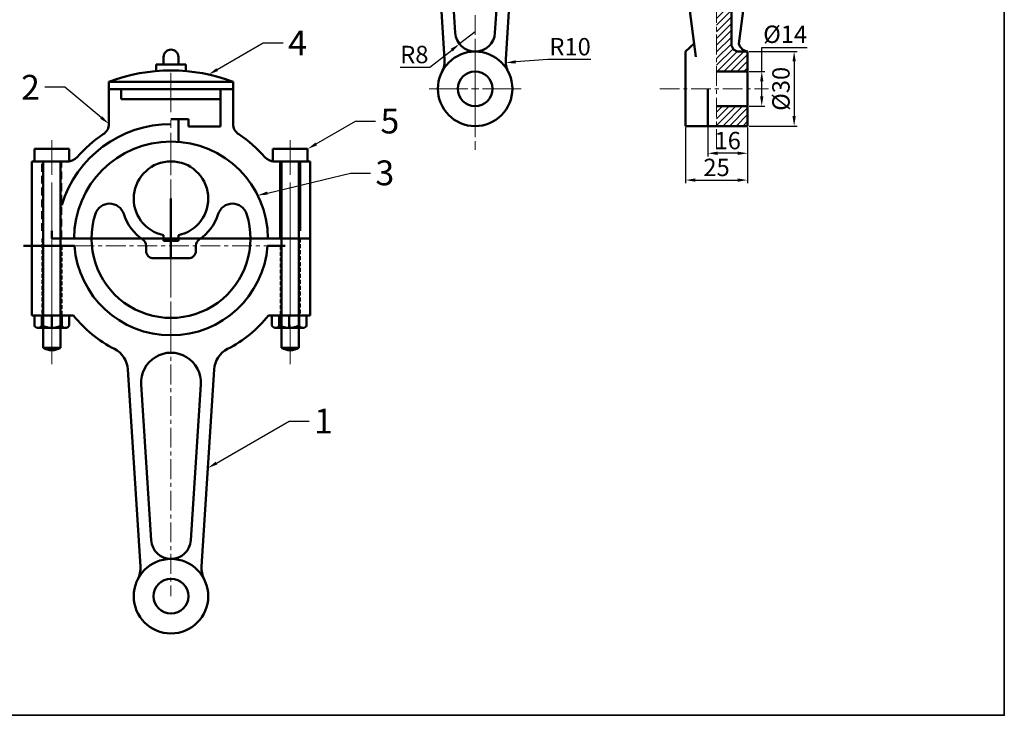
# Model space of a CAD drawing. Units: millimetres. Extents: x 214 to 813, y -258 to 321.
# Tile 2 of 4: x 416 to 813, y -258 to 22. Entities that reach past the tile are written whole.
import ezdxf
from ezdxf import colors
from ezdxf.entities.mleader import LeaderData, LeaderLine
from ezdxf.math import Vec2, Vec3

# ---------------------------------------------------------------- set-up
doc = ezdxf.new("R2010")
doc.units = ezdxf.units.MM
doc.header["$LTSCALE"] = 0.5
doc.linetypes.add('CENTER', pattern=[50.8, 31.75, -6.35, 6.35, -6.35])
doc.linetypes.add('HIDDEN', pattern=[9.525, 6.35, -3.175])
for name, color, linetype, lineweight in [('M-CNTR', 1, 'CENTER', 18), ('M-DIMS', 2, 'Continuous', 25), ('M-HATC', 8, 'Continuous', 18), ('M-HIDN', 6, 'HIDDEN', 25), ('M-OUTL', 7, 'Continuous', 50), ('M-TTLB', 7, 'Continuous', 35)]:
    doc.layers.add(name, color=color, linetype=linetype, lineweight=lineweight)
doc.styles.get("Standard").update_dxf_attribs({"font": 'arial.ttf'})
doc.dimstyles.new('ISO-25', dxfattribs={"dimtxt": 7, "dimasz": 4, "dimexe": 1.25, "dimexo": 0.625, "dimtad": 1, "dimtoh": 1, "dimtxsty": 'Standard', "dimcen": 2.5, "dimadec": 0, "dimazin": 0, "dimtfac": 1, "dimtmove": 0, "dimatfit": 3, "dimfxl": 1, "dimarcsym": 0})

# ---------------------------------------------------------------- blocks, each defined once
blk = doc.blocks.new('*U2')
at = {"layer": 'M-CNTR', "color": 0, "transparency": 16777216}
for p, q in [((0, 7.8), (0, 42.5)), ((-42.5, 0), (-7.8, 0)), ((7.8, 0), (42.5, 0)), ((0, -42.5), (0, -7.8))]:
    blk.add_line(p, q, dxfattribs=at)
at = {"layer": 'M-CNTR', "color": 0, "linetype": 'Continuous', "transparency": 16777216}
for p, q in [((-3.9, 0), (3.9, 0)), ((0, -3.9), (0, 3.9))]:
    blk.add_line(p, q, dxfattribs=at)
blk = doc.blocks.new('*D23')
at = {"layer": 'Defpoints', "color": 0, "ltscale": 0.5, "transparency": 16777216}
for p in [(599.66, 17.04), (593.37, 12.1)]:
    blk.add_point(p, dxfattribs=at)
at = {"layer": 'M-DIMS', "color": 0, "lineweight": -2, "ltscale": 0.5, "transparency": 16777216}
for p, q in [((599.66, 17.04), (593.37, 12.1)), ((581.46, 2.74), (590.23, 9.63)), ((569.54, 2.74), (581.46, 2.74))]:
    blk.add_line(p, q, dxfattribs=at)
at = {"layer": 'M-DIMS', "color": 0, "ltscale": 0.5, "transparency": 16777216}
blk.add_solid([(589.82, 10.15), (590.64, 9.1), (593.37, 12.1)], dxfattribs=at)
at = {"layer": 'M-DIMS', "color": 0, "ltscale": 0.5, "transparency": 16777216, "insert": (575.19, 6.94), "char_height": 7, "attachment_point": 5}
blk.add_mtext('R8', dxfattribs=at)
blk = doc.blocks.new('*D24')
at = {"layer": 'Defpoints', "color": 0, "ltscale": 0.5, "transparency": 16777216}
for p in [(612, 4.55), (621.97, 5.34)]:
    blk.add_point(p, dxfattribs=at)
at = {"layer": 'M-DIMS', "color": 0, "lineweight": -2, "ltscale": 0.5, "transparency": 16777216}
for p, q in [((628.92, 5.89), (615.99, 4.87)), ((646.25, 5.89), (628.92, 5.89))]:
    blk.add_line(p, q, dxfattribs=at)
at = {"layer": 'M-DIMS', "color": 0, "ltscale": 0.5, "transparency": 16777216}
blk.add_solid([(615.93, 5.53), (616.04, 4.2), (612, 4.55)], dxfattribs=at)
at = {"layer": 'M-DIMS', "color": 0, "ltscale": 0.5, "transparency": 16777216, "insert": (637.9, 10.09), "char_height": 7, "attachment_point": 5}
blk.add_mtext('R10', dxfattribs=at)
blk = doc.blocks.new('*U25')
at = {"layer": 'M-CNTR', "color": 0, "transparency": 16777216}
for p, q in [((0, 3), (0, 18.5)), ((-18.5, 0), (-3, 0)), ((3, 0), (18.5, 0)), ((0, -18.5), (0, -3))]:
    blk.add_line(p, q, dxfattribs=at)
at = {"layer": 'M-CNTR', "color": 0, "linetype": 'Continuous', "transparency": 16777216}
for p, q in [((-1.5, 0), (1.5, 0)), ((0, -1.5), (0, 1.5))]:
    blk.add_line(p, q, dxfattribs=at)
blk = doc.blocks.new('*U39')
at = {"layer": 'M-CNTR', "color": 0, "transparency": 16777216}
blk.add_line((0, -84.16), (0, 6), dxfattribs=at)
blk = doc.blocks.new('*D62')
at = {"layer": 'Defpoints', "color": 0, "ltscale": 0.5, "transparency": 16777216}
for p in [(709.36, 1.04), (709.36, -12.96), (715.07, -12.96)]:
    blk.add_point(p, dxfattribs=at)
at = {"layer": 'M-DIMS', "color": 0, "lineweight": -2, "ltscale": 0.5, "transparency": 16777216}
for p, q in [((715.07, 1.04), (715.07, 10.7)), ((715.07, 10.7), (733.31, 10.7)), ((709.99, 1.04), (716.32, 1.04)), ((715.07, -8.96), (715.07, -2.96)), ((709.99, -12.96), (716.32, -12.96))]:
    blk.add_line(p, q, dxfattribs=at)
at = {"layer": 'M-DIMS', "color": 0, "ltscale": 0.5, "transparency": 16777216}
for points in [[(714.4, -2.96), (715.73, -2.96), (715.07, 1.04)], [(714.4, -8.96), (715.73, -8.96), (715.07, -12.96)]]:
    blk.add_solid(points, dxfattribs=at)
at = {"layer": 'M-DIMS', "color": 0, "ltscale": 0.5, "transparency": 16777216, "insert": (724.5, 15.09), "char_height": 7, "attachment_point": 5}
blk.add_mtext('%%C14', dxfattribs=at)
blk = doc.blocks.new('*D63')
at = {"layer": 'Defpoints', "color": 0, "ltscale": 0.5, "transparency": 16777216}
for p in [(709.36, 9.04), (709.36, -20.96), (728.1, -20.96)]:
    blk.add_point(p, dxfattribs=at)
at = {"layer": 'M-DIMS', "color": 0, "lineweight": -2, "ltscale": 0.5, "transparency": 16777216}
for p, q in [((709.99, 9.04), (729.35, 9.04)), ((728.1, 5.04), (728.1, -16.96)), ((709.99, -20.96), (729.35, -20.96))]:
    blk.add_line(p, q, dxfattribs=at)
at = {"layer": 'M-DIMS', "color": 0, "ltscale": 0.5, "transparency": 16777216}
for points in [[(727.43, 5.04), (728.76, 5.04), (728.1, 9.04)], [(727.43, -16.96), (728.76, -16.96), (728.1, -20.96)]]:
    blk.add_solid(points, dxfattribs=at)
at = {"layer": 'M-DIMS', "color": 0, "ltscale": 0.5, "transparency": 16777216, "insert": (723.7, -5.96), "char_height": 7, "attachment_point": 5, "rotation": 90}
blk.add_mtext('%%C30', dxfattribs=at)
blk = doc.blocks.new('*D64')
at = {"layer": 'Defpoints', "color": 0, "ltscale": 0.5, "transparency": 16777216}
for p in [(693.36, -20.96), (709.36, -20.96), (693.36, -31.9)]:
    blk.add_point(p, dxfattribs=at)
at = {"layer": 'M-DIMS', "color": 0, "lineweight": -2, "ltscale": 0.5, "transparency": 16777216}
for p, q in [((693.36, -21.58), (693.36, -33.15)), ((709.36, -21.58), (709.36, -33.15)), ((705.36, -31.9), (697.36, -31.9))]:
    blk.add_line(p, q, dxfattribs=at)
at = {"layer": 'M-DIMS', "color": 0, "ltscale": 0.5, "transparency": 16777216}
for points in [[(697.36, -31.23), (697.36, -32.57), (693.36, -31.9)], [(705.36, -31.23), (705.36, -32.57), (709.36, -31.9)]]:
    blk.add_solid(points, dxfattribs=at)
at = {"layer": 'M-DIMS', "color": 0, "ltscale": 0.5, "transparency": 16777216, "insert": (701.36, -27.7), "char_height": 7, "attachment_point": 5}
blk.add_mtext('16', dxfattribs=at)
blk = doc.blocks.new('*D65')
at = {"layer": 'Defpoints', "color": 0, "ltscale": 0.5, "transparency": 16777216}
for p in [(684.36, -20.96), (709.36, -20.96), (709.36, -42.69)]:
    blk.add_point(p, dxfattribs=at)
at = {"layer": 'M-DIMS', "color": 0, "lineweight": -2, "ltscale": 0.5, "transparency": 16777216}
for p, q in [((684.36, -21.58), (684.36, -43.94)), ((709.36, -21.58), (709.36, -43.94)), ((688.36, -42.69), (705.36, -42.69))]:
    blk.add_line(p, q, dxfattribs=at)
at = {"layer": 'M-DIMS', "color": 0, "ltscale": 0.5, "transparency": 16777216}
for points in [[(688.36, -42.03), (688.36, -43.36), (684.36, -42.69)], [(705.36, -42.03), (705.36, -43.36), (709.36, -42.69)]]:
    blk.add_solid(points, dxfattribs=at)
at = {"layer": 'M-DIMS', "color": 0, "ltscale": 0.5, "transparency": 16777216, "insert": (696.86, -38.49), "char_height": 7, "attachment_point": 5}
blk.add_mtext('25', dxfattribs=at)
blk = doc.blocks.new('*U69')
at = {"layer": 'M-CNTR', "color": 0, "transparency": 16777216}
blk.add_line((0, -84.16), (0, 6), dxfattribs=at)
blk = doc.blocks.new('ECCENTRIC-SHEAVE-WEB')
at = {"ltscale": 0.5}
for p, q in [((32, 48), (32, 24)), ((22, 27), (22, 29.03)), ((42, 27), (42, 29.03)), ((32, 24), (25, 24)), ((32, 24), (39, 24))]:
    blk.add_line(p, q, dxfattribs=at)
for centre, radius, start, end in [((7.26, 40), 6, 17.9202, 162.0798), ((56.74, 40), 6, 17.9202, 162.0798), ((32, 32), 32, 162.0798, 17.9202), ((32, 48), 20, 197.9202, 235.5826), ((32, 48), 20, 304.4174, 342.0798), ((19, 29.03), 3, 0, 55.5826), ((45, 29.03), 3, 124.4174, 180), ((25, 27), 3, 180, 270), ((39, 27), 3, 270, 0)]:
    blk.add_arc(centre, radius, start, end, dxfattribs=at)
blk = doc.blocks.new('BOLT-HEAD')
at = {"ltscale": 0.5}
for p, q in [((14, 5), (0, 5)), ((0, 5), (0, 0)), ((14, 0), (14, 5)), ((0, 0), (14, 0))]:
    blk.add_line(p, q, dxfattribs=at)

msp = doc.modelspace()

# ---------------------------------------------------------------- hatches: boundary and pattern name
at = {"layer": 'M-HATC', "ltscale": 0.5}
h = msp.add_hatch(dxfattribs=at)
h.set_pattern_fill('ANSI31', color=256, scale=0.6)
h.set_pattern_definition([(45, (-63.675, 1e-14), (-1.3470384, 1.3470384), [])])
h.paths.add_polyline_path([(696.86, 1.042), (709.36, 1.042), (709.36, 9.042), (705.86, 9.042, -0.4142136), (702.86, 12.042), (702.86, 89.042, -0.4142136), (705.86, 92.042), (717.86, 92.042), (717.86, 99.042), (696.86, 99.042), (696.86, 92.042)])
h.paths.add_polyline_path([(696.86, -12.958), (696.86, -20.958), (709.36, -20.958), (709.36, -12.958)])

# ---------------------------------------------------------------- linework, layer by layer
at = {"layer": 'M-CNTR', "ltscale": 0.5}
for p, q in [((599.664, 138.042), (599.664, -30.466)), ((696.86, 92.042), (696.86, -31.942)), ((673.979, -5.958), (717.766, -5.958)), ((429.217, -66.162), (429.217, -97.162)), ((477.217, -66.162), (477.217, -210.162)), ((525.217, -66.162), (525.217, -97.162)), ((438.333, -69.162), (516.102, -69.162))]:
    msp.add_line(p, q, dxfattribs=at)
at = {"layer": 'M-CNTR'}
for p, q in [((477.217, -66.162), (477.217, 1.587)), ((429.217, -84.881), (429.217, -28.818)), ((525.217, -84.881), (525.217, -28.818))]:
    msp.add_line(p, q, dxfattribs=at)
at = {"layer": 'M-HIDN'}
for p, q in [((425.217, -63.162), (425.217, -35.162)), ((433.217, -66.162), (433.217, -35.162))]:
    msp.add_line(p, q, dxfattribs=at)
at = {"layer": 'M-HIDN', "ltscale": 0.5}
for p, q in [((425.217, -66.162), (425.217, -97.162)), ((529.217, -66.162), (529.217, -97.162)), ((433.217, -69.162), (433.217, -97.162)), ((521.217, -69.162), (521.217, -97.162))]:
    msp.add_line(p, q, dxfattribs=at)
at = {"layer": 'M-OUTL', "ltscale": 0.5}
for p, q in [((676.438, 99.042), (688.528, 6.956)), ((702.86, 89.042), (702.86, 12.042)), ((715.923, 88.687), (705.87, 12.115)), ((582.297, 85.272), (587.342, 5.974)), ((617.031, 85.272), (611.986, 5.974)), ((587.689, 79.28), (591.68, 16.534)), ((611.64, 79.28), (607.648, 16.534)), ((684.36, 9.042), (687.824, 12.315)), ((684.36, -20.958), (684.36, 9.042)), ((705.86, 9.042), (709.36, 9.042)), ((709.36, 9.042), (709.36, -20.958)), ((474.217, 6.838), (474.217, 3.838)), ((480.217, 3.838), (480.217, 6.838)), ((471.217, 3.838), (483.217, 3.838)), ((471.217, 3.838), (471.217, 1.197)), ((483.217, 3.838), (483.217, 1.197)), ((709.36, 1.042), (696.86, 1.042)), ((452.217, -6.162), (452.217, -3.162)), ((452.217, -3.162), (502.217, -3.162)), ((502.217, -3.162), (502.217, -6.162)), ((457.217, -6.162), (452.217, -6.162)), ((457.217, -10.162), (457.217, -6.162)), ((457.217, -6.162), (497.217, -6.162)), ((497.217, -6.162), (497.217, -10.162)), ((502.217, -6.162), (497.217, -6.162)), ((693.36, -20.958), (693.36, -5.958)), ((477.217, -10.162), (457.217, -10.162)), ((497.217, -10.162), (477.217, -10.162)), ((709.36, -12.958), (696.86, -12.958)), ((709.36, -20.958), (684.36, -20.958)), ((425.717, -35.162), (425.717, -110.162)), ((432.717, -110.162), (432.717, -35.162)), ((521.717, -35.162), (521.717, -110.162)), ((528.717, -110.162), (528.717, -35.162)), ((421.217, -66.162), (421.217, -97.162)), ((431.217, -66.162), (429.217, -66.162)), ((477.217, -66.162), (469.33, -66.162)), ((474.217, -67.162), (474.217, -64.859)), ((480.217, -67.162), (474.217, -67.162)), ((480.217, -64.859), (480.217, -67.162)), ((523.217, -66.162), (533.217, -66.162)), ((533.217, -66.162), (533.217, -97.162)), ((431.315, -69.162), (417.892, -69.162)), ((438.333, -69.162), (431.217, -69.162)), ((516.102, -69.162), (523.119, -69.162)), ((437.987, -97.162), (421.217, -97.162)), ((436.217, -97.162), (422.217, -97.162)), ((422.217, -97.162), (422.217, -101.162)), ((425.217, -97.162), (425.217, -101.162)), ((429.217, -97.162), (429.217, -102.162)), ((433.217, -97.162), (433.217, -101.162)), ((436.217, -101.162), (436.217, -97.162)), ((516.447, -97.162), (533.217, -97.162)), ((531.832, -97.162), (517.832, -97.162)), ((517.832, -97.162), (517.832, -101.162)), ((520.832, -97.162), (520.832, -101.162)), ((524.832, -97.162), (524.832, -102.162)), ((528.832, -97.162), (528.832, -101.162)), ((531.832, -101.162), (531.832, -97.162)), ((423.685, -102.162), (434.851, -102.162)), ((519.3, -102.162), (530.466, -102.162)), ((425.717, -110.162), (432.717, -110.162)), ((521.717, -110.162), (528.717, -110.162)), ((459.85, -118.933), (464.895, -198.23)), ((494.584, -118.933), (489.539, -198.23)), ((465.241, -124.924), (469.233, -187.67)), ((489.193, -124.924), (485.201, -187.67))]:
    msp.add_line(p, q, dxfattribs=at)
at = {"layer": 'M-OUTL'}
for p, q in [((452.217, -6.162), (502.217, -6.162)), ((452.217, -6.162), (452.217, -20.064)), ((497.217, -6.162), (497.217, -21.162)), ((502.217, -6.162), (502.217, -20.064)), ((484.217, -18.162), (477.217, -18.162)), ((480.217, -27.278), (480.217, -18.162)), ((484.217, -21.162), (484.217, -18.162)), ((497.217, -21.162), (484.217, -21.162)), ((435.636, -35.162), (421.217, -35.162)), ((421.217, -66.162), (421.217, -35.162)), ((518.798, -35.162), (533.217, -35.162)), ((521.217, -66.162), (521.217, -35.162)), ((529.217, -63.162), (529.217, -35.162)), ((533.217, -66.162), (533.217, -35.162)), ((429.217, -66.162), (429.217, -63.162)), ((527.217, -66.162), (429.217, -66.162))]:
    msp.add_line(p, q, dxfattribs=at)
at = {"layer": 'M-OUTL', "ltscale": 0.5}
for centre, radius in [((599.664, -5.958), 15), ((599.664, -5.958), 7), ((477.217, -210.162), 15), ((477.217, -210.162), 7)]:
    msp.add_circle(centre, radius, dxfattribs=at)
for centre, radius, start, end in [((599.664, 17.042), 8, 183.64028, 356.35972), ((705.86, 12.042), 3, 180, 270), ((709.991, 13.278), 4.283, 195.7658, 261.52495), ((477.217, 6.838), 3, 0, 180), ((577.362, 5.339), 10, 333.13555, 3.64028), ((621.966, 5.339), 10, 176.35972, 206.86445), ((477.217, -68.546), 70, 69.07517, 110.92483), ((477.217, -50.162), 15, 281.53696, 258.46304), ((477.217, -66.162), 39, 184.41173, 355.58827), ((477.217, -66.162), 50, 218.31613, 242.88477), ((477.217, -66.162), 50, 297.11523, 321.68387), ((423.717, -100.538), 1.625, 202.60314, 337.39686), ((429.217, -93.662), 8.5, 241.92751, 298.07249), ((434.717, -100.546), 1.622, 202.32738, 337.67261), ((519.332, -100.538), 1.625, 202.60314, 337.39686), ((524.832, -93.662), 8.5, 241.92751, 298.07249), ((530.332, -100.546), 1.622, 202.32738, 337.67261), ((429.217, -104.423), 6.722, 238.62157, 301.37843), ((449.87, -119.568), 10, 3.64028, 62.88477), ((504.564, -119.568), 10, 117.11523, 176.35972), ((525.217, -104.423), 6.722, 238.62157, 301.37843), ((477.217, -124.162), 12, 356.35972, 183.64028), ((477.217, -187.162), 8, 183.64028, 356.35972), ((454.915, -198.865), 10, 333.13555, 3.64028), ((499.519, -198.865), 10, 176.35972, 206.86445)]:
    msp.add_arc(centre, radius, start, end, dxfattribs=at)
at = {"layer": 'M-OUTL'}
for centre, radius, start, end in [((477.217, -66.162), 46, 90, 163.04257), ((447.217, -20.064), 5, 303.05573, 0), ((507.217, -20.064), 5, 180, 236.94427), ((477.217, -66.162), 39, 0, 180), ((477.217, -66.162), 50, 123.05573, 139.11481), ((477.217, -66.162), 50, 40.88519, 56.94427), ((435.636, -30.162), 5, 270, 319.11481), ((518.798, -30.162), 5, 220.88519, 270)]:
    msp.add_arc(centre, radius, start, end, dxfattribs=at)
at = {"layer": 'M-TTLB', "ltscale": 0.5}
msp.add_lwpolyline([(214.186, 321.5), (812.717, 321.5), (812.717, -258.089), (214.186, -258.089)], close=True, dxfattribs=at)

# ---------------------------------------------------------------- block references
at = {"layer": 'M-CNTR'}
for name, p in [('*U25', (599.664, -5.958)), ('*U2', (477.217, -66.162)), ('*U39', (429.217, -32.662)), ('*U69', (525.217, -32.662))]:
    msp.add_blockref(name, p, dxfattribs=at)
at = {"layer": 'M-OUTL'}
for name, p in [('BOLT-HEAD', (422.218, -35.162)), ('BOLT-HEAD', (518.218, -35.162)), ('ECCENTRIC-SHEAVE-WEB', (445.216, -98.162))]:
    msp.add_blockref(name, p, dxfattribs=at)

# ---------------------------------------------------------------- dimensions: what is measured, and where the dimension line sits
at = {"layer": 'M-DIMS', "ltscale": 0.5}
dim = msp.add_linear_dim(base=(715.068, -12.958), p1=(709.36, 1.042), p2=(709.36, -12.958), angle=90, text='%%C<>', dimstyle='ISO-25', override={"dimclrd": 0, "dimclre": 0, "dimclrt": 0}, dxfattribs=at)
dim.commit()
dim.dimension.update_dxf_attribs({"geometry": '*D62', "text_midpoint": (724.5, 10.698), "dimtype": 160})
dim = msp.add_radius_dim(center=(599.664, 17.042), mpoint=(593.374, 12.1), dimstyle='ISO-25', override={"dimclrd": 0, "dimclre": 0, "dimclrt": 0}, dxfattribs=at)
dim.commit()
dim.dimension.update_dxf_attribs({"geometry": '*D23', "text_midpoint": (575.187, 6.94)})
dim = msp.add_radius_dim(center=(621.966, 5.339), mpoint=(611.998, 4.549), dimstyle='ISO-25', override={"dimclrd": 0, "dimclre": 0, "dimclrt": 0}, dxfattribs=at)
dim.commit()
dim.dimension.update_dxf_attribs({"geometry": '*D24', "text_midpoint": (628.921, 5.891), "dimtype": 164})
dim = msp.add_linear_dim(base=(728.098, -20.958), p1=(709.36, 9.042), p2=(709.36, -20.958), angle=90, text='%%C<>', dimstyle='ISO-25', override={"dimclrd": 0, "dimclre": 0, "dimclrt": 0}, dxfattribs=at)
dim.commit()
dim.dimension.update_dxf_attribs({"geometry": '*D63', "text_midpoint": (723.703, -5.958)})
for base, p1, p2, picture, middle in [((709.36, -42.693), (684.36, -20.958), (709.36, -20.958), '*D65', (696.86, -38.494)), ((693.36, -31.899), (709.36, -20.958), (693.36, -20.958), '*D64', (701.36, -27.7))]:
    dim = msp.add_linear_dim(base=base, p1=p1, p2=p2, dimstyle='ISO-25', override={"dimclrd": 0, "dimclre": 0, "dimclrt": 0}, dxfattribs=at)
    dim.commit()
    dim.dimension.update_dxf_attribs({"geometry": picture, "text_midpoint": middle})

# ---------------------------------------------------------------- leaders
ml = msp.add_multileader_mtext('Standard', dxfattribs=at)
ml.set_content('4', color=256)
ml.set_leader_properties()
ml.build(insert=Vec2(0, 0))
ctx = ml.context
ctx.base_point, ctx.char_height, ctx.plane_origin = Vec3(522.367, 12.493), 10, Vec3(492.372, -0.206)
notes = []
notes.append((ctx, [(0, (1, 1, 0), (514.367, 12.493), (1, 0), 8, [(0, [(492.372, -0.206)], 0, [])])]))
ctx.mtext.insert, ctx.mtext.flow_direction = Vec3(524.367, 17.493), 5
ml = msp.add_multileader_mtext('Standard', dxfattribs=at)
ml.set_content('2', color=256)
ml.set_leader_properties()
ml.build(insert=Vec2(0, 0))
ctx = ml.context
ctx.base_point, ctx.char_height, ctx.plane_origin = Vec3(415.809, -5.351), 10, Vec3(452.217, -20.064)
ctx.text_align_type = 2
notes.append((ctx, [(0, (1, 1, 0), (434.432, -5.351), (-1, 0), 8, [(0, [(452.217, -20.064)], 0, [])])]))
ctx.mtext.insert, ctx.mtext.alignment, ctx.mtext.flow_direction = Vec3(424.432, -0.351), 3, 5
ml = msp.add_multileader_mtext('Standard', dxfattribs=at)
ml.set_content('5', color=256)
ml.set_leader_properties()
ml.build(insert=Vec2(0, 0))
ctx = ml.context
ctx.base_point, ctx.char_height, ctx.plane_origin = Vec3(559.556, -18.996), 10, Vec3(532.217, -30.162)
notes.append((ctx, [(0, (1, 1, 0), (551.556, -18.996), (1, 0), 8, [(0, [(532.217, -30.162)], 0, [])])]))
ctx.mtext.insert, ctx.mtext.flow_direction = Vec3(561.556, -13.911), 5
ml = msp.add_multileader_mtext('Standard', dxfattribs=at)
ml.set_content('3', color=256)
ml.set_leader_properties()
ml.build(insert=Vec2(0, 0))
ctx = ml.context
ctx.base_point, ctx.char_height, ctx.plane_origin = Vec3(557.52, -39.864), 10, Vec3(512.163, -48.848)
notes.append((ctx, [(0, (1, 1, 0), (549.52, -39.864), (1, 0), 8, [(0, [(512.163, -48.848)], 0, [])])]))
ctx.mtext.insert, ctx.mtext.flow_direction = Vec3(559.52, -34.775), 5
ml = msp.add_multileader_mtext('Standard', dxfattribs=at)
ml.set_content('1', color=256)
ml.set_leader_properties()
ml.build(insert=Vec2(0, 0))
ctx = ml.context
ctx.base_point, ctx.char_height, ctx.plane_origin = Vec3(532.83, -139.662), 10, Vec3(492.062, -158.581)
notes.append((ctx, [(0, (1, 1, 0), (524.83, -139.662), (1, 0), 8, [(0, [(492.062, -158.581)], 0, [])])]))
ctx.mtext.insert, ctx.mtext.flow_direction = Vec3(534.83, -134.662), 5
for ctx, leaders in notes:
    for number, flags, end, landing, length, lines in leaders:
        leader = LeaderData()
        leader.index, (leader.has_last_leader_line, leader.has_dogleg_vector, leader.attachment_direction) = number, flags
        leader.last_leader_point, leader.dogleg_vector, leader.dogleg_length = Vec3(end), Vec3(landing), length
        for number, points, colour, breaks in lines:
            line = LeaderLine()
            line.index, line.vertices, line.color, line.breaks = number, Vec3.list(points), colors.encode_raw_color(colour), breaks
            leader.lines.append(line)
        ctx.leaders.append(leader)

doc.saveas('drawing.dxf')
